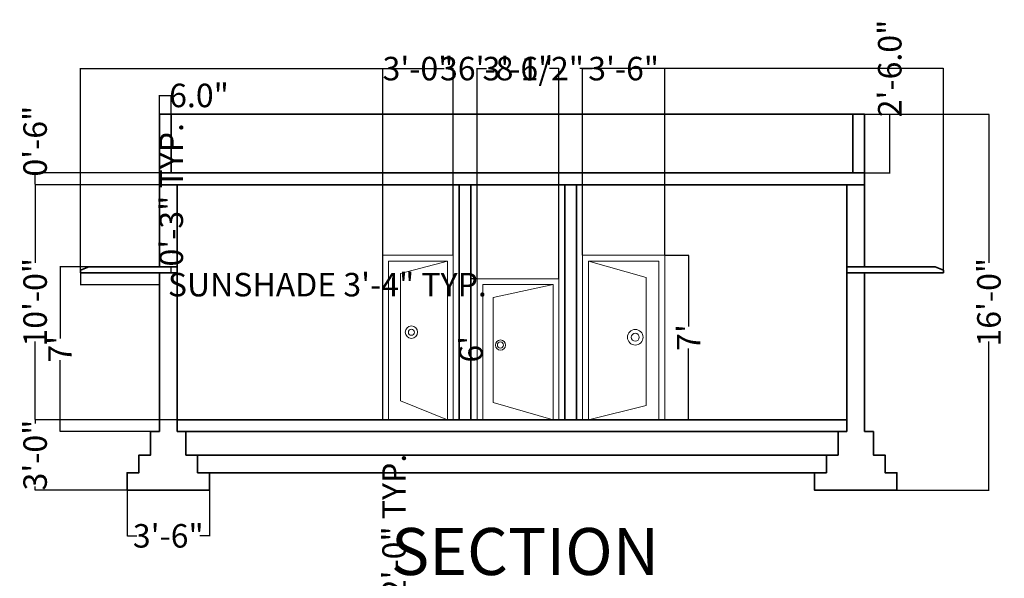
# Model space of a CAD drawing. Units: inches. Extents: x -91 to 1027, y -85 to 599.
# Tile 3 of 3: x 508 to 1011, y 248 to 533. Entities that reach past the tile are written whole.
import ezdxf

# ---------------------------------------------------------------- set-up
doc = ezdxf.new("R2010")
doc.units = ezdxf.units.IN
doc.header["$MEASUREMENT"] = 0
for name, color, linetype, lineweight in [('A-ANNO-DIMS', 2, 'Continuous', 18), ('A-ANNO-TEXT', 7, 'Continuous', 35), ('A-SECT-DOOR', 3, 'Continuous', 18), ('A-SECT-FLOR', 7, 'Continuous', 35), ('A-SECT-ROOF', 7, 'Continuous', 35), ('A-SECT-WALL', 7, 'Continuous', 35), ('S-FNDN', 1, 'Continuous', 35)]:
    doc.layers.add(name, color=color, linetype=linetype, lineweight=lineweight)
doc.styles.get("Standard").update_dxf_attribs({"font": 'arial.ttf'})
doc.dimstyles.get("Standard").update_dxf_attribs({"dimtxt": 12, "dimasz": 0.18, "dimexe": 0.18, "dimexo": 0.0625, "dimgap": 0.09, "dimtad": 0, "dimdec": 1, "dimzin": 0, "dimdsep": 46, "dimlunit": 3, "dimtxsty": 'Standard', "dimcen": 0.09, "dimadec": 0, "dimazin": 0, "dimtfac": 1, "dimtdec": 1, "dimtofl": 0, "dimtmove": 0, "dimatfit": 3, "dimfxl": 1, "dimtolj": 1, "dimtzin": 0, "dimarcsym": 0})

# ---------------------------------------------------------------- blocks, each defined once
blk = doc.blocks.new('*D5')
at = {"layer": 'A-ANNO-DIMS', "color": 0, "lineweight": -2, "transparency": 16777216}
for p, q in [((837.65, 412.52), (849.94, 412.52)), ((849.76, 412.34), (849.76, 376.09)), ((849.76, 328.7), (849.76, 364.96)), ((837.65, 328.52), (849.94, 328.52))]:
    blk.add_line(p, q, dxfattribs=at)
at = {"layer": 'A-ANNO-DIMS', "color": 0, "transparency": 16777216}
for points in [[(849.73, 412.34), (849.79, 412.34), (849.76, 412.52)], [(849.73, 328.7), (849.79, 328.7), (849.76, 328.52)]]:
    blk.add_solid(points, dxfattribs=at)
at = {"layer": 'Defpoints', "color": 0, "transparency": 16777216}
for p in [(837.58, 412.52), (849.76, 412.52), (837.58, 328.52)]:
    blk.add_point(p, dxfattribs=at)
at = {"layer": 'A-ANNO-DIMS', "color": 0, "transparency": 16777216, "insert": (849.76, 370.52), "char_height": 12, "attachment_point": 5, "rotation": 90}
blk.add_mtext("\\A1;7'", dxfattribs=at)
blk = doc.blocks.new('*D6')
at = {"layer": 'A-ANNO-DIMS', "color": 0, "lineweight": -2, "transparency": 16777216}
for p, q in [((741.66, 400.52), (738.4, 400.52)), ((738.58, 400.34), (738.58, 370.17)), ((738.58, 328.7), (738.58, 358.88)), ((741.66, 328.52), (738.4, 328.52))]:
    blk.add_line(p, q, dxfattribs=at)
at = {"layer": 'A-ANNO-DIMS', "color": 0, "transparency": 16777216}
for points in [[(738.55, 400.34), (738.61, 400.34), (738.58, 400.52)], [(738.55, 328.7), (738.61, 328.7), (738.58, 328.52)]]:
    blk.add_solid(points, dxfattribs=at)
at = {"layer": 'Defpoints', "color": 0, "transparency": 16777216}
for p in [(738.58, 400.52), (741.72, 400.52), (741.72, 328.52)]:
    blk.add_point(p, dxfattribs=at)
at = {"layer": 'A-ANNO-DIMS', "color": 0, "transparency": 16777216, "insert": (738.58, 364.52), "char_height": 12, "attachment_point": 5, "rotation": 90}
blk.add_mtext("\\A1;6'", dxfattribs=at)
blk = doc.blocks.new('*D7')
at = {"layer": 'A-ANNO-DIMS', "color": 0, "lineweight": -2, "transparency": 16777216}
for p, q in [((579.52, 406.52), (528.63, 406.52)), ((528.81, 406.34), (528.81, 370.09)), ((528.81, 322.7), (528.81, 358.96)), ((579.52, 322.52), (528.63, 322.52))]:
    blk.add_line(p, q, dxfattribs=at)
at = {"layer": 'A-ANNO-DIMS', "color": 0, "transparency": 16777216}
for points in [[(528.78, 406.34), (528.84, 406.34), (528.81, 406.52)], [(528.78, 322.7), (528.84, 322.7), (528.81, 322.52)]]:
    blk.add_solid(points, dxfattribs=at)
at = {"layer": 'Defpoints', "color": 0, "transparency": 16777216}
for p in [(528.81, 406.52), (579.58, 406.52), (579.58, 322.52)]:
    blk.add_point(p, dxfattribs=at)
at = {"layer": 'A-ANNO-DIMS', "color": 0, "transparency": 16777216, "insert": (528.81, 364.52), "char_height": 12, "attachment_point": 5, "rotation": 90}
blk.add_mtext("\\A1;7'", dxfattribs=at)
blk = doc.blocks.new('*D8')
at = {"layer": 'A-ANNO-DIMS', "color": 0, "lineweight": -2, "transparency": 16777216}
for p, q in [((939.65, 484.52), (952.65, 484.52)), ((952.47, 484.52), (952.47, 484.7)), ((952.47, 454.7), (952.47, 484.34)), ((939.65, 454.52), (952.65, 454.52))]:
    blk.add_line(p, q, dxfattribs=at)
at = {"layer": 'A-ANNO-DIMS', "color": 0, "transparency": 16777216}
for points in [[(952.44, 484.34), (952.5, 484.34), (952.47, 484.52)], [(952.44, 454.7), (952.5, 454.7), (952.47, 454.52)]]:
    blk.add_solid(points, dxfattribs=at)
at = {"layer": 'Defpoints', "color": 0, "transparency": 16777216}
for p in [(939.58, 484.52), (952.47, 484.52), (939.58, 454.52)]:
    blk.add_point(p, dxfattribs=at)
at = {"layer": 'A-ANNO-DIMS', "color": 0, "transparency": 16777216, "insert": (952.47, 507.84), "char_height": 12, "attachment_point": 5, "rotation": 90}
blk.add_mtext('\\A1;2\'-6.0"', dxfattribs=at)
blk = doc.blocks.new('*D16')
at = {"layer": 'A-ANNO-DIMS', "color": 0, "lineweight": -2, "transparency": 16777216}
for p, q in [((579.58, 473.51), (579.58, 494.25)), ((579.76, 494.07), (585.4, 494.07)), ((585.58, 473.51), (585.58, 494.25)), ((585.58, 494.07), (585.76, 494.07))]:
    blk.add_line(p, q, dxfattribs=at)
at = {"layer": 'A-ANNO-DIMS', "color": 0, "transparency": 16777216}
for points in [[(579.76, 494.1), (579.76, 494.04), (579.58, 494.07)], [(585.4, 494.1), (585.4, 494.04), (585.58, 494.07)]]:
    blk.add_solid(points, dxfattribs=at)
at = {"layer": 'Defpoints', "color": 0, "transparency": 16777216}
for p in [(585.58, 494.07), (579.58, 473.45), (585.58, 473.45)]:
    blk.add_point(p, dxfattribs=at)
at = {"layer": 'A-ANNO-DIMS', "color": 0, "transparency": 16777216, "insert": (599.77, 494.07), "char_height": 12, "attachment_point": 5}
blk.add_mtext('\\A1;6.0"', dxfattribs=at)
blk = doc.blocks.new('SUNSHADE-SECTION')
for p, q in [((0, 1.39), (4.25, 3)), ((0, 0), (0, 1.39)), ((40.25, 3), (4.25, 3)), ((4.25, 0), (0, 0)), ((4.25, 0), (40.25, 0))]:
    blk.add_line(p, q)
blk = doc.blocks.new('*D30')
at = {"layer": 'A-ANNO-DIMS', "color": 0, "lineweight": -2, "transparency": 16777216}
for p, q in [((702.92, 181.03), (699.16, 181.03)), ((699.34, 181.03), (699.34, 181.21)), ((699.34, 156.99), (699.34, 180.85)), ((702.92, 156.81), (699.16, 156.81))]:
    blk.add_line(p, q, dxfattribs=at)
at = {"layer": 'A-ANNO-DIMS', "color": 0, "transparency": 16777216}
for points in [[(699.31, 180.85), (699.37, 180.85), (699.34, 181.03)], [(699.31, 156.99), (699.37, 156.99), (699.34, 156.81)]]:
    blk.add_solid(points, dxfattribs=at)
at = {"layer": 'Defpoints', "color": 0, "transparency": 16777216}
for p in [(699.34, 181.03), (702.98, 181.03), (702.98, 156.81)]:
    blk.add_point(p, dxfattribs=at)
at = {"layer": 'A-ANNO-DIMS', "color": 0, "transparency": 16777216, "insert": (699.34, 247.39), "char_height": 12, "attachment_point": 5, "rotation": 90}
blk.add_mtext('\\A1;PANEL 2\'-0" TYP.', dxfattribs=at)
blk = doc.blocks.new('*D32')
at = {"layer": 'A-ANNO-DIMS', "color": 0, "lineweight": -2, "transparency": 16777216}
for p, q in [((539.34, 403.46), (539.34, 397.31)), ((579.58, 403.46), (579.58, 397.31)), ((539.52, 397.49), (579.4, 397.49)), ((579.58, 397.49), (579.76, 397.49))]:
    blk.add_line(p, q, dxfattribs=at)
at = {"layer": 'A-ANNO-DIMS', "color": 0, "transparency": 16777216}
for points in [[(539.52, 397.52), (539.52, 397.46), (539.34, 397.49)], [(579.4, 397.52), (579.4, 397.46), (579.58, 397.49)]]:
    blk.add_solid(points, dxfattribs=at)
at = {"layer": 'Defpoints', "color": 0, "transparency": 16777216}
for p in [(539.34, 403.52), (579.58, 403.52), (579.58, 397.49)]:
    blk.add_point(p, dxfattribs=at)
at = {"layer": 'A-ANNO-DIMS', "color": 0, "transparency": 16777216, "insert": (665.3, 397.49), "char_height": 12, "attachment_point": 5}
blk.add_mtext('\\A1;SUNSHADE 3\'-4" TYP.', dxfattribs=at)
blk = doc.blocks.new('*D33')
at = {"layer": 'A-ANNO-DIMS', "color": 0, "lineweight": -2, "transparency": 16777216}
for p, q in [((579.65, 406.52), (585.8, 406.52)), ((579.65, 403.52), (585.8, 403.52)), ((585.62, 406.52), (585.62, 406.7)), ((585.62, 403.7), (585.62, 406.34))]:
    blk.add_line(p, q, dxfattribs=at)
at = {"layer": 'A-ANNO-DIMS', "color": 0, "transparency": 16777216}
for points in [[(585.59, 406.34), (585.65, 406.34), (585.62, 406.52)], [(585.59, 403.7), (585.65, 403.7), (585.62, 403.52)]]:
    blk.add_solid(points, dxfattribs=at)
at = {"layer": 'Defpoints', "color": 0, "transparency": 16777216}
for p in [(579.58, 406.52), (579.58, 403.52), (585.62, 406.52)]:
    blk.add_point(p, dxfattribs=at)
at = {"layer": 'A-ANNO-DIMS', "color": 0, "transparency": 16777216, "insert": (585.62, 443.37), "char_height": 12, "attachment_point": 5, "rotation": 90}
blk.add_mtext('\\A1;0\'-3" TYP.', dxfattribs=at)
blk = doc.blocks.new('*D53')
at = {"layer": 'A-ANNO-DIMS', "color": 0, "lineweight": -2, "transparency": 16777216}
for p, q in [((539.34, 404.97), (539.34, 507.95)), ((539.52, 507.77), (724.9, 507.77)), ((979.65, 507.77), (794.26, 507.77)), ((979.83, 404.96), (979.83, 507.95))]:
    blk.add_line(p, q, dxfattribs=at)
at = {"layer": 'A-ANNO-DIMS', "color": 0, "transparency": 16777216}
for points in [[(539.52, 507.8), (539.52, 507.74), (539.34, 507.77)], [(979.65, 507.8), (979.65, 507.74), (979.83, 507.77)]]:
    blk.add_solid(points, dxfattribs=at)
at = {"layer": 'Defpoints', "color": 0, "transparency": 16777216}
for p in [(979.83, 507.77), (539.34, 404.91), (979.83, 404.9)]:
    blk.add_point(p, dxfattribs=at)
at = {"layer": 'A-ANNO-DIMS', "color": 0, "transparency": 16777216, "insert": (759.58, 507.77), "char_height": 12, "attachment_point": 5}
blk.add_mtext('\\A1;36\'-8 1/2"', dxfattribs=at)
blk = doc.blocks.new('*D54')
at = {"layer": 'A-ANNO-DIMS', "color": 0, "lineweight": -2, "transparency": 16777216}
for p, q in [((939.65, 484.52), (1003.26, 484.52)), ((1003.08, 484.34), (1003.08, 408.66)), ((1003.08, 292.7), (1003.08, 368.39)), ((956.15, 292.52), (1003.26, 292.52))]:
    blk.add_line(p, q, dxfattribs=at)
at = {"layer": 'A-ANNO-DIMS', "color": 0, "transparency": 16777216}
for points in [[(1003.05, 484.34), (1003.11, 484.34), (1003.08, 484.52)], [(1003.05, 292.7), (1003.11, 292.7), (1003.08, 292.52)]]:
    blk.add_solid(points, dxfattribs=at)
at = {"layer": 'Defpoints', "color": 0, "transparency": 16777216}
for p in [(939.58, 484.52), (956.08, 292.52), (1003.08, 292.52)]:
    blk.add_point(p, dxfattribs=at)
at = {"layer": 'A-ANNO-DIMS', "color": 0, "transparency": 16777216, "insert": (1003.08, 388.52), "char_height": 12, "attachment_point": 5, "rotation": 90}
blk.add_mtext('\\A1;16\'-0"', dxfattribs=at)
blk = doc.blocks.new('*D55')
at = {"layer": 'A-ANNO-DIMS', "color": 0, "lineweight": -2, "transparency": 16777216}
for p, q in [((588.52, 448.52), (515.91, 448.52)), ((516.09, 448.34), (516.09, 408.66)), ((516.09, 328.7), (516.09, 368.39)), ((588.52, 328.52), (515.91, 328.52))]:
    blk.add_line(p, q, dxfattribs=at)
at = {"layer": 'A-ANNO-DIMS', "color": 0, "transparency": 16777216}
for points in [[(516.06, 448.34), (516.12, 448.34), (516.09, 448.52)], [(516.06, 328.7), (516.12, 328.7), (516.09, 328.52)]]:
    blk.add_solid(points, dxfattribs=at)
at = {"layer": 'Defpoints', "color": 0, "transparency": 16777216}
for p in [(516.09, 448.52), (588.58, 448.52), (588.58, 328.52)]:
    blk.add_point(p, dxfattribs=at)
at = {"layer": 'A-ANNO-DIMS', "color": 0, "transparency": 16777216, "insert": (516.09, 388.52), "char_height": 12, "attachment_point": 5, "rotation": 90}
blk.add_mtext('\\A1;10\'-0"', dxfattribs=at)
blk = doc.blocks.new('*D56')
at = {"layer": 'A-ANNO-DIMS', "color": 0, "lineweight": -2, "transparency": 16777216}
for p, q in [((579.52, 454.52), (515.91, 454.52)), ((516.09, 454.52), (516.09, 454.7)), ((516.09, 448.7), (516.09, 454.34)), ((579.52, 448.52), (515.91, 448.52))]:
    blk.add_line(p, q, dxfattribs=at)
at = {"layer": 'A-ANNO-DIMS', "color": 0, "transparency": 16777216}
for points in [[(516.06, 454.34), (516.12, 454.34), (516.09, 454.52)], [(516.06, 448.7), (516.12, 448.7), (516.09, 448.52)]]:
    blk.add_solid(points, dxfattribs=at)
at = {"layer": 'Defpoints', "color": 0, "transparency": 16777216}
for p in [(516.09, 454.52), (579.58, 454.52), (579.58, 448.52)]:
    blk.add_point(p, dxfattribs=at)
at = {"layer": 'A-ANNO-DIMS', "color": 0, "transparency": 16777216, "insert": (516.09, 470.74), "char_height": 12, "attachment_point": 5, "rotation": 90}
blk.add_mtext('\\A1;0\'-6"', dxfattribs=at)
blk = doc.blocks.new('*D57')
at = {"layer": 'A-ANNO-DIMS', "color": 0, "lineweight": -2, "transparency": 16777216}
for p, q in [((563.08, 292.46), (563.08, 269.09)), ((605.08, 292.46), (605.08, 269.09)), ((563.26, 269.27), (568.05, 269.27)), ((604.9, 269.27), (600.12, 269.27))]:
    blk.add_line(p, q, dxfattribs=at)
at = {"layer": 'A-ANNO-DIMS', "color": 0, "transparency": 16777216}
for points in [[(563.26, 269.3), (563.26, 269.24), (563.08, 269.27)], [(604.9, 269.3), (604.9, 269.24), (605.08, 269.27)]]:
    blk.add_solid(points, dxfattribs=at)
at = {"layer": 'Defpoints', "color": 0, "transparency": 16777216}
for p in [(563.08, 292.52), (605.08, 292.52), (605.08, 269.27)]:
    blk.add_point(p, dxfattribs=at)
at = {"layer": 'A-ANNO-DIMS', "color": 0, "transparency": 16777216, "insert": (584.08, 269.27), "char_height": 12, "attachment_point": 5}
blk.add_mtext('\\A1;3\'-6"', dxfattribs=at)
blk = doc.blocks.new('*D58')
at = {"layer": 'A-ANNO-DIMS', "color": 0, "lineweight": -2, "transparency": 16777216}
for p, q in [((588.52, 328.52), (515.91, 328.52)), ((516.09, 328.34), (516.09, 326.56)), ((563.02, 292.52), (515.91, 292.52)), ((516.09, 292.7), (516.09, 294.49))]:
    blk.add_line(p, q, dxfattribs=at)
at = {"layer": 'A-ANNO-DIMS', "color": 0, "transparency": 16777216}
for points in [[(516.06, 328.34), (516.12, 328.34), (516.09, 328.52)], [(516.06, 292.7), (516.12, 292.7), (516.09, 292.52)]]:
    blk.add_solid(points, dxfattribs=at)
at = {"layer": 'Defpoints', "color": 0, "transparency": 16777216}
for p in [(516.09, 328.52), (588.58, 328.52), (563.08, 292.52)]:
    blk.add_point(p, dxfattribs=at)
at = {"layer": 'A-ANNO-DIMS', "color": 0, "transparency": 16777216, "insert": (516.09, 310.52), "char_height": 12, "attachment_point": 5, "rotation": 90}
blk.add_mtext('\\A1;3\'-0"', dxfattribs=at)
blk = doc.blocks.new('*D59')
at = {"layer": 'A-ANNO-DIMS', "color": 0, "lineweight": -2, "transparency": 16777216}
for p, q in [((693.55, 412.59), (693.55, 507.95)), ((693.73, 507.77), (695.54, 507.77)), ((729.43, 507.77), (727.61, 507.77)), ((729.61, 412.59), (729.61, 507.95))]:
    blk.add_line(p, q, dxfattribs=at)
at = {"layer": 'A-ANNO-DIMS', "color": 0, "transparency": 16777216}
for points in [[(693.73, 507.8), (693.73, 507.74), (693.55, 507.77)], [(729.43, 507.8), (729.43, 507.74), (729.61, 507.77)]]:
    blk.add_solid(points, dxfattribs=at)
at = {"layer": 'Defpoints', "color": 0, "transparency": 16777216}
for p in [(729.61, 507.77), (693.55, 412.52), (729.61, 412.52)]:
    blk.add_point(p, dxfattribs=at)
at = {"layer": 'A-ANNO-DIMS', "color": 0, "transparency": 16777216, "insert": (711.58, 507.77), "char_height": 12, "attachment_point": 5}
blk.add_mtext('\\A1;3\'-0"', dxfattribs=at)
blk = doc.blocks.new('*D60')
at = {"layer": 'A-ANNO-DIMS', "color": 0, "lineweight": -2, "transparency": 16777216}
for p, q in [((741.72, 400.59), (741.72, 507.95)), ((741.9, 507.77), (746.58, 507.77)), ((783.34, 507.77), (778.66, 507.77)), ((783.52, 400.59), (783.52, 507.95))]:
    blk.add_line(p, q, dxfattribs=at)
at = {"layer": 'A-ANNO-DIMS', "color": 0, "transparency": 16777216}
for points in [[(741.9, 507.8), (741.9, 507.74), (741.72, 507.77)], [(783.34, 507.8), (783.34, 507.74), (783.52, 507.77)]]:
    blk.add_solid(points, dxfattribs=at)
at = {"layer": 'Defpoints', "color": 0, "transparency": 16777216}
for p in [(783.52, 507.77), (741.72, 400.52), (783.52, 400.52)]:
    blk.add_point(p, dxfattribs=at)
at = {"layer": 'A-ANNO-DIMS', "color": 0, "transparency": 16777216, "insert": (762.62, 507.77), "char_height": 12, "attachment_point": 5}
blk.add_mtext('\\A1;3\'-6"', dxfattribs=at)
blk = doc.blocks.new('*D61')
at = {"layer": 'A-ANNO-DIMS', "color": 0, "lineweight": -2, "transparency": 16777216}
for p, q in [((795.58, 412.59), (795.58, 507.95)), ((795.76, 507.77), (800.55, 507.77)), ((837.4, 507.77), (832.62, 507.77)), ((837.58, 412.59), (837.58, 507.95))]:
    blk.add_line(p, q, dxfattribs=at)
at = {"layer": 'A-ANNO-DIMS', "color": 0, "transparency": 16777216}
for points in [[(795.76, 507.8), (795.76, 507.74), (795.58, 507.77)], [(837.4, 507.8), (837.4, 507.74), (837.58, 507.77)]]:
    blk.add_solid(points, dxfattribs=at)
at = {"layer": 'Defpoints', "color": 0, "transparency": 16777216}
for p in [(837.58, 507.77), (795.58, 412.52), (837.58, 412.52)]:
    blk.add_point(p, dxfattribs=at)
at = {"layer": 'A-ANNO-DIMS', "color": 0, "transparency": 16777216, "insert": (816.58, 507.77), "char_height": 12, "attachment_point": 5}
blk.add_mtext('\\A1;3\'-6"', dxfattribs=at)

msp = doc.modelspace()

# ---------------------------------------------------------------- linework, layer by layer
at = {"layer": 'A-SECT-DOOR'}
for p, q in [((693.55, 328.52), (693.55, 412.52)), ((729.48, 412.52), (729.48, 328.52)), ((795.58, 412.52), (795.58, 328.52)), ((837.58, 412.52), (837.58, 328.52)), ((726.61, 409.52), (702.7, 403.13)), ((798.58, 409.52), (828.13, 401.14)), ((702.7, 403.13), (702.7, 338.25)), ((693.54, 400.52), (693.55, 400.52)), ((729.48, 400.52), (729.61, 400.52)), ((780.52, 397.52), (749.89, 390.85)), ((828.13, 401.14), (828.13, 335.89)), ((749.89, 390.85), (749.89, 337.4)), ((702.7, 338.25), (726.61, 328.52)), ((749.89, 337.4), (780.52, 328.52)), ((828.13, 335.89), (798.58, 328.52))]:
    msp.add_line(p, q, dxfattribs=at)
for points in [[(693.54, 328.52), (693.54, 412.52), (729.61, 412.52), (729.61, 328.52)], [(795.58, 328.52), (795.58, 412.52), (837.58, 412.52), (837.58, 328.52)], [(696.54, 328.52), (696.54, 409.52), (726.61, 409.52), (726.61, 328.52)], [(798.58, 328.52), (798.58, 409.52), (834.58, 409.52), (834.58, 328.52)], [(741.72, 328.52), (741.72, 400.52), (783.52, 400.52), (783.52, 328.52)], [(744.72, 328.52), (744.72, 397.52), (780.52, 397.52), (780.52, 328.52)]]:
    msp.add_lwpolyline(points, dxfattribs=at)
for centre, radius in [((708.22, 373.22), 3.17), ((708.22, 373.22), 3.17), ((708.22, 373.22), 1.55), ((822.51, 370.64), 3.97), ((822.51, 370.64), 3.97), ((822.51, 370.64), 2.06), ((753.69, 366.67), 2.6), ((753.69, 366.67), 1.59)]:
    msp.add_circle(centre, radius, dxfattribs=at)
at = {"layer": 'A-SECT-FLOR'}
for p, q in [((588.58, 328.52), (930.58, 328.52)), ((588.58, 322.52), (930.58, 322.52))]:
    msp.add_line(p, q, dxfattribs=at)
at = {"layer": 'A-SECT-ROOF'}
for p, q in [((579.58, 484.52), (939.58, 484.52)), ((585.58, 454.52), (585.58, 484.52)), ((933.58, 484.52), (933.58, 454.52)), ((579.58, 454.52), (939.58, 454.52)), ((579.58, 448.52), (939.58, 448.52)), ((579.58, 406.52), (588.61, 406.52)), ((579.58, 403.52), (588.61, 403.52)), ((939.58, 406.51), (930.58, 406.51)), ((939.58, 403.51), (930.58, 403.51))]:
    msp.add_line(p, q, dxfattribs=at)
at = {"layer": 'A-SECT-WALL'}
for p, q in [((579.58, 406.52), (579.58, 484.52)), ((939.58, 484.52), (939.58, 406.51)), ((579.58, 448.52), (579.58, 406.52)), ((588.58, 322.52), (588.58, 448.52)), ((588.61, 448.52), (588.61, 328.52)), ((732.53, 448.52), (732.53, 328.52)), ((732.58, 328.52), (732.58, 448.52)), ((738.58, 448.52), (738.58, 328.52)), ((738.58, 328.52), (738.58, 448.52)), ((786.58, 448.52), (786.58, 328.52)), ((786.58, 328.52), (786.58, 448.52)), ((792.58, 448.52), (792.58, 328.52)), ((792.58, 328.52), (792.58, 448.52)), ((930.58, 448.52), (930.58, 322.52)), ((732.53, 412.52), (732.58, 412.52)), ((579.58, 322.52), (579.58, 403.52)), ((579.58, 403.52), (579.58, 328.52)), ((939.58, 403.51), (939.58, 322.52)), ((732.53, 400.52), (732.58, 400.52))]:
    msp.add_line(p, q, dxfattribs=at)
at = {"layer": 'S-FNDN'}
for p, q in [((599.08, 310.52), (920.08, 310.52)), ((914.08, 301.52), (605.08, 301.52))]:
    msp.add_line(p, q, dxfattribs=at)
for points in [[(579.58, 322.52), (575.08, 322.52), (575.08, 310.52), (569.08, 310.52), (569.08, 301.52), (563.08, 301.52), (563.08, 292.52), (605.08, 292.52), (605.08, 301.52), (599.08, 301.52), (599.08, 310.52), (593.08, 310.52), (593.08, 322.52), (588.58, 322.52)], [(939.58, 322.52), (944.08, 322.52), (944.08, 310.52), (950.08, 310.52), (950.08, 301.52), (956.08, 301.52), (956.08, 292.52), (914.08, 292.52), (914.08, 301.52), (920.08, 301.52), (920.08, 310.52), (926.08, 310.52), (926.08, 322.52), (930.58, 322.52)]]:
    msp.add_lwpolyline(points, dxfattribs=at)

# ---------------------------------------------------------------- block references
at = {"layer": 'A-SECT-ROOF'}
msp.add_blockref('SUNSHADE-SECTION', (539.34, 403.52), dxfattribs=at)
at = {"layer": 'A-SECT-ROOF', "extrusion": (0, 0, -1), "zscale": -1, "rotation": 0.0027392291971345}
msp.add_blockref('SUNSHADE-SECTION', (-979.83, 403.51), dxfattribs=at)

# ---------------------------------------------------------------- texts
at = {"layer": 'A-ANNO-TEXT'}
msp.add_text('SECTION', height=24, dxfattribs=at).set_placement((697.83, 249.28))

# ---------------------------------------------------------------- dimensions: what is measured, and where the dimension line sits
at = {"layer": 'A-ANNO-DIMS'}
for base, p1, p2, override, picture, middle in [((952.47, 484.52), (939.58, 454.52), (939.58, 484.52), {"dimclrd": 0, "dimclre": 0, "dimclrt": 0}, '*D8', (952.47, 507.84)), ((516.09, 454.52), (579.58, 448.52), (579.58, 454.52), {"dimdec": 1, "dimlfac": 1, "dimrnd": 0, "dimzin": 1, "dimdsep": 46, "dimlunit": 4, "dimfrac": 2}, '*D56', (516.09, 470.74)), ((1003.08, 292.52), (939.58, 484.52), (956.08, 292.52), {"dimdec": 1, "dimlfac": 1, "dimrnd": 0, "dimzin": 1, "dimdsep": 46, "dimlunit": 4, "dimfrac": 2}, '*D54', (1003.08, 388.52)), ((516.09, 448.52), (588.58, 328.52), (588.58, 448.52), {"dimdec": 1, "dimlfac": 1, "dimrnd": 0, "dimzin": 1, "dimdsep": 46, "dimlunit": 4, "dimfrac": 2}, '*D55', (516.09, 388.52)), ((849.76, 412.52), (837.58, 328.52), (837.58, 412.52), {"dimclrd": 0, "dimclre": 0, "dimclrt": 0}, '*D5', (849.76, 370.52)), ((528.81, 406.52), (579.58, 322.52), (579.58, 406.52), {"dimclrd": 0, "dimclre": 0, "dimclrt": 0}, '*D7', (528.81, 364.52)), ((738.58, 400.52), (741.72, 328.52), (741.72, 400.52), {"dimclrd": 0, "dimclre": 0, "dimclrt": 0}, '*D6', (738.58, 364.52)), ((516.09, 328.52), (563.08, 292.52), (588.58, 328.52), {"dimdec": 1, "dimlfac": 1, "dimrnd": 0, "dimzin": 1, "dimdsep": 46, "dimlunit": 4, "dimfrac": 2}, '*D58', (516.09, 310.52))]:
    dim = msp.add_linear_dim(base=base, p1=p1, p2=p2, angle=90, dimstyle='Standard', override=override, dxfattribs=at)
    dim.commit()
    dim.dimension.update_dxf_attribs({"geometry": picture, "text_midpoint": middle})
for base, p1, p2, override, picture, middle in [((979.83, 507.77), (539.34, 404.91), (979.83, 404.9), {"dimdec": 1, "dimlfac": 1, "dimrnd": 0, "dimzin": 1, "dimdsep": 46, "dimlunit": 4, "dimfrac": 2}, '*D53', (759.58, 507.77)), ((729.61, 507.77), (693.55, 412.52), (729.61, 412.52), {"dimdec": 1, "dimlfac": 1, "dimrnd": 0, "dimzin": 1, "dimdsep": 46, "dimlunit": 4, "dimfrac": 2}, '*D59', (711.58, 507.77)), ((783.52, 507.77), (741.72, 400.52), (783.52, 400.52), {"dimdec": 1, "dimlfac": 1, "dimrnd": 0, "dimzin": 1, "dimdsep": 46, "dimlunit": 4, "dimfrac": 2}, '*D60', (762.62, 507.77)), ((837.58, 507.77), (795.58, 412.52), (837.58, 412.52), {"dimdec": 1, "dimlfac": 1, "dimrnd": 0, "dimzin": 1, "dimdsep": 46, "dimlunit": 4, "dimfrac": 2}, '*D61', (816.58, 507.77)), ((585.58, 494.07), (579.58, 473.45), (585.58, 473.45), {"dimclrd": 0, "dimclre": 0, "dimclrt": 0}, '*D16', (599.77, 494.07)), ((605.08, 269.27), (563.08, 292.52), (605.08, 292.52), {"dimdec": 1, "dimlfac": 1, "dimrnd": 0, "dimzin": 1, "dimdsep": 46, "dimlunit": 4, "dimfrac": 2}, '*D57', (584.08, 269.27))]:
    dim = msp.add_linear_dim(base=base, p1=p1, p2=p2, dimstyle='Standard', override=override, dxfattribs=at)
    dim.commit()
    dim.dimension.update_dxf_attribs({"geometry": picture, "text_midpoint": middle})
for base, p1, p2, text, picture, middle in [((585.62, 406.52), (579.58, 403.52), (579.58, 406.52), '<> TYP.', '*D33', (585.62, 443.37)), ((699.34, 181.03), (702.98, 156.81), (702.98, 181.03), 'PANEL <> TYP.', '*D30', (699.34, 247.39))]:
    dim = msp.add_linear_dim(base=base, p1=p1, p2=p2, angle=90, text=text, dimstyle='Standard', override={"dimdec": 1, "dimlfac": 1, "dimrnd": 0, "dimzin": 1, "dimdsep": 46, "dimlunit": 4, "dimfrac": 2}, dxfattribs=at)
    dim.commit()
    dim.dimension.update_dxf_attribs({"geometry": picture, "text_midpoint": middle})
dim = msp.add_linear_dim(base=(579.58, 397.49), p1=(539.34, 403.52), p2=(579.58, 403.52), text='SUNSHADE <> TYP.', dimstyle='Standard', override={"dimdec": 1, "dimlfac": 1, "dimrnd": 0, "dimzin": 1, "dimdsep": 46, "dimlunit": 4, "dimfrac": 2}, dxfattribs=at)
dim.commit()
dim.dimension.update_dxf_attribs({"geometry": '*D32', "text_midpoint": (665.3, 397.49)})

doc.saveas('drawing.dxf')
